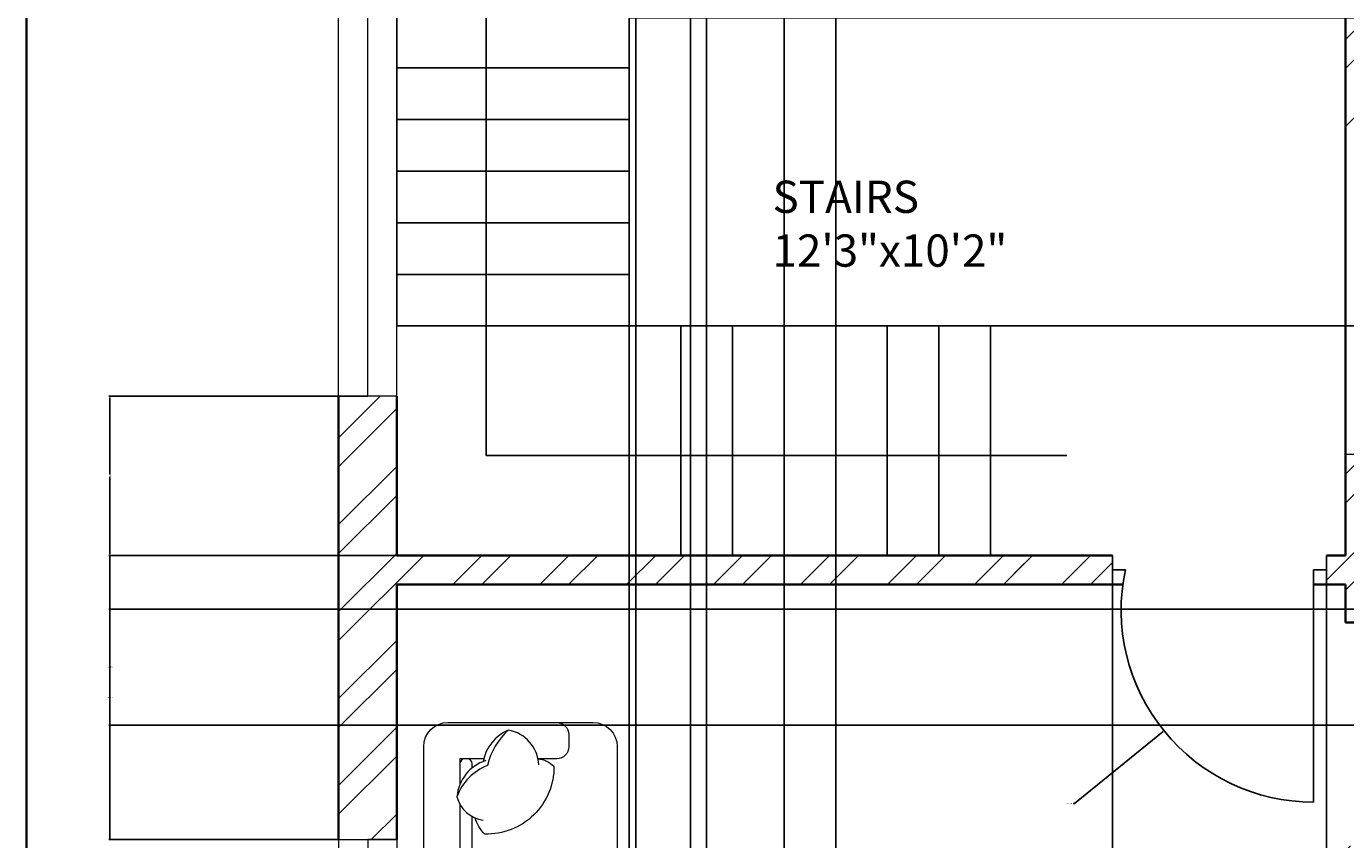
# Model space of a CAD drawing. Units: inches. Extents: x 2529 to 3014, y 1203 to 2262.
# Tile 3 of 13: x 2529 to 2733, y 1747 to 1873. Entities that reach past the tile are written whole.
import ezdxf

# ---------------------------------------------------------------- set-up
doc = ezdxf.new("R2010")
doc.units = ezdxf.units.IN
for name, color, linetype, lineweight in [('A-ANNO-DIMS', 2, 'Continuous', 18), ('A-ANNO-TTLB', 7, 'Continuous', 35), ('A-AREA-IDEN', 7, 'Continuous', 18), ('A-DOOR', 21, 'Continuous', 25), ('A-FLOR-STRS', 61, 'Continuous', 25), ('A-FURN', 8, 'Continuous', 18), ('A-GLAZ', 191, 'Continuous', 18), ('A-WALL', 7, 'Continuous', 35), ('A-WALL-PATT', 143, 'Continuous', 13)]:
    doc.layers.add(name, color=color, linetype=linetype, lineweight=lineweight)
doc.styles.get("Standard").update_dxf_attribs({"font": 'arial.ttf'})
doc.dimstyles.get("Standard").update_dxf_attribs({"dimtxt": 0.18, "dimasz": 0.18, "dimexe": 0.18, "dimexo": 0.0625, "dimgap": 0.09, "dimtad": 0, "dimtih": 1, "dimtoh": 1, "dimdec": 4, "dimzin": 0, "dimdsep": 46, "dimtxsty": 'Standard', "dimcen": 0.09, "dimadec": 0, "dimazin": 0, "dimtfac": 1, "dimtdec": 4, "dimtofl": 0, "dimtmove": 0, "dimatfit": 3, "dimfxl": 1, "dimtolj": 1, "dimtzin": 0, "dimarcsym": 0})

# ---------------------------------------------------------------- blocks, each defined once
blk = doc.blocks.new('WIN-60x9')
for p, q in [((0, 60), (9, 60)), ((0, 60), (0, 0)), ((9, 60), (4.5, 60)), ((4.5, 60), (4.5, 0)), ((9, 60), (9, 0)), ((4.5, 0), (0, 0)), ((0, 0), (9, 0))]:
    blk.add_line(p, q)
blk = doc.blocks.new('*D23')
at = {"layer": 'A-ANNO-DIMS', "color": 0, "lineweight": -2, "transparency": 16777216}
for p, q in [((2585.99, 1791), (2541.45, 1791)), ((2541.63, 1790.82), (2541.63, 1769.16)), ((2541.63, 1747.13), (2541.63, 1768.79)), ((2576.99, 1746.95), (2541.45, 1746.95))]:
    blk.add_line(p, q, dxfattribs=at)
at = {"layer": 'A-ANNO-DIMS', "color": 0, "transparency": 16777216}
for points in [[(2541.6, 1790.82), (2541.66, 1790.82), (2541.63, 1791)], [(2541.6, 1747.13), (2541.66, 1747.13), (2541.63, 1746.95)]]:
    blk.add_solid(points, dxfattribs=at)
at = {"layer": 'Defpoints', "color": 0, "transparency": 16777216}
for p in [(2541.63, 1791), (2586.06, 1791), (2577.06, 1746.95)]:
    blk.add_point(p, dxfattribs=at)
at = {"layer": 'A-ANNO-DIMS', "color": 0, "transparency": 16777216, "insert": (2541.63, 1768.98), "char_height": 0.18, "attachment_point": 5}
blk.add_mtext('\\A1;44.055', dxfattribs=at)
blk = doc.blocks.new('*D24')
at = {"layer": 'A-ANNO-DIMS', "color": 0, "lineweight": -2, "transparency": 16777216}
for p, q in [((2576.99, 1815.67), (2541.45, 1815.67)), ((2541.63, 1815.49), (2541.63, 1803.52)), ((2541.63, 1791.18), (2541.63, 1803.16)), ((2585.99, 1791), (2541.45, 1791))]:
    blk.add_line(p, q, dxfattribs=at)
at = {"layer": 'A-ANNO-DIMS', "color": 0, "transparency": 16777216}
for points in [[(2541.6, 1815.49), (2541.66, 1815.49), (2541.63, 1815.67)], [(2541.6, 1791.18), (2541.66, 1791.18), (2541.63, 1791)]]:
    blk.add_solid(points, dxfattribs=at)
at = {"layer": 'Defpoints', "color": 0, "transparency": 16777216}
for p in [(2541.63, 1815.67), (2577.06, 1815.67), (2586.06, 1791)]:
    blk.add_point(p, dxfattribs=at)
at = {"layer": 'A-ANNO-DIMS', "color": 0, "transparency": 16777216, "insert": (2541.63, 1803.34), "char_height": 0.18, "attachment_point": 5}
blk.add_mtext('\\A1;24.67', dxfattribs=at)
blk = doc.blocks.new('*D32')
at = {"layer": 'A-ANNO-DIMS', "color": 0, "lineweight": -2, "transparency": 16777216}
for p, q in [((2586.06, 1826.63), (2586.06, 2243.11)), ((2586.24, 2242.93), (2603.84, 2242.93)), ((2621.88, 2242.93), (2604.27, 2242.93)), ((2622.06, 1826.63), (2622.06, 2243.11))]:
    blk.add_line(p, q, dxfattribs=at)
at = {"layer": 'A-ANNO-DIMS', "color": 0, "transparency": 16777216}
for points in [[(2586.24, 2242.96), (2586.24, 2242.9), (2586.06, 2242.93)], [(2621.88, 2242.96), (2621.88, 2242.9), (2622.06, 2242.93)]]:
    blk.add_solid(points, dxfattribs=at)
at = {"layer": 'Defpoints', "color": 0, "transparency": 16777216}
for p in [(2622.06, 2242.93), (2586.06, 1826.57), (2622.06, 1826.57)]:
    blk.add_point(p, dxfattribs=at)
at = {"layer": 'A-ANNO-DIMS', "color": 0, "transparency": 16777216, "insert": (2604.06, 2242.93), "char_height": 0.18, "attachment_point": 5}
blk.add_mtext('\\A1;36', dxfattribs=at)
blk = doc.blocks.new('*D53')
at = {"layer": 'A-ANNO-DIMS', "color": 0, "lineweight": -2, "transparency": 16777216}
for p, q in [((2696.93, 1790.94), (2696.93, 1483.77)), ((2730.09, 1790.94), (2730.09, 1483.77)), ((2697.11, 1483.95), (2713.11, 1483.95)), ((2729.91, 1483.95), (2713.9, 1483.95))]:
    blk.add_line(p, q, dxfattribs=at)
at = {"layer": 'A-ANNO-DIMS', "color": 0, "transparency": 16777216}
for points in [[(2697.11, 1483.98), (2697.11, 1483.92), (2696.93, 1483.95)], [(2729.91, 1483.98), (2729.91, 1483.92), (2730.09, 1483.95)]]:
    blk.add_solid(points, dxfattribs=at)
at = {"layer": 'Defpoints', "color": 0, "transparency": 16777216}
for p in [(2696.93, 1791), (2730.09, 1791), (2730.09, 1483.95)]:
    blk.add_point(p, dxfattribs=at)
at = {"layer": 'A-ANNO-DIMS', "color": 0, "transparency": 16777216, "insert": (2713.51, 1483.95), "char_height": 0.18, "attachment_point": 5}
blk.add_mtext('\\A1;33.15', dxfattribs=at)
blk = doc.blocks.new('*D62')
at = {"layer": 'A-ANNO-DIMS', "color": 0, "lineweight": -2, "transparency": 16777216}
for p, q in [((2904.99, 1782.69), (2541.45, 1782.69)), ((2541.63, 1782.51), (2541.63, 1773.88)), ((2541.63, 1764.89), (2541.63, 1773.52)), ((2904.99, 1764.71), (2541.45, 1764.71))]:
    blk.add_line(p, q, dxfattribs=at)
at = {"layer": 'A-ANNO-DIMS', "color": 0, "transparency": 16777216}
for points in [[(2541.6, 1782.51), (2541.66, 1782.51), (2541.63, 1782.69)], [(2541.6, 1764.89), (2541.66, 1764.89), (2541.63, 1764.71)]]:
    blk.add_solid(points, dxfattribs=at)
at = {"layer": 'Defpoints', "color": 0, "transparency": 16777216}
for p in [(2905.06, 1782.69), (2541.63, 1764.71), (2905.06, 1764.71)]:
    blk.add_point(p, dxfattribs=at)
at = {"layer": 'A-ANNO-DIMS', "color": 0, "transparency": 16777216, "insert": (2541.63, 1773.7), "char_height": 0.18, "attachment_point": 5}
blk.add_mtext('\\A1;17.983', dxfattribs=at)
blk = doc.blocks.new('*D65')
at = {"layer": 'A-ANNO-DIMS', "color": 0, "lineweight": -2, "transparency": 16777216}
for p, q in [((2646.06, 1874.24), (2646.06, 1483.77)), ((2654.06, 1874.24), (2654.06, 1483.77)), ((2646.24, 1483.95), (2649.91, 1483.95)), ((2653.88, 1483.95), (2650.2, 1483.95))]:
    blk.add_line(p, q, dxfattribs=at)
at = {"layer": 'A-ANNO-DIMS', "color": 0, "transparency": 16777216}
for points in [[(2646.24, 1483.98), (2646.24, 1483.92), (2646.06, 1483.95)], [(2653.88, 1483.98), (2653.88, 1483.92), (2654.06, 1483.95)]]:
    blk.add_solid(points, dxfattribs=at)
at = {"layer": 'Defpoints', "color": 0, "transparency": 16777216}
for p in [(2646.06, 1874.3), (2654.06, 1874.3), (2654.06, 1483.95)]:
    blk.add_point(p, dxfattribs=at)
at = {"layer": 'A-ANNO-DIMS', "color": 0, "transparency": 16777216, "insert": (2650.06, 1483.95), "char_height": 0.18, "attachment_point": 5}
blk.add_mtext('\\A1;8', dxfattribs=at)
blk = doc.blocks.new('*D68')
at = {"layer": 'A-ANNO-DIMS', "color": 0, "lineweight": -2, "transparency": 16777216}
for p, q in [((2622.12, 1874.3), (3007.66, 1874.3)), ((3007.48, 1874.12), (3007.48, 1850.62)), ((3007.48, 1826.75), (3007.48, 1850.25)), ((2622.12, 1826.57), (3007.66, 1826.57))]:
    blk.add_line(p, q, dxfattribs=at)
at = {"layer": 'A-ANNO-DIMS', "color": 0, "transparency": 16777216}
for points in [[(3007.45, 1874.12), (3007.51, 1874.12), (3007.48, 1874.3)], [(3007.45, 1826.75), (3007.51, 1826.75), (3007.48, 1826.57)]]:
    blk.add_solid(points, dxfattribs=at)
at = {"layer": 'Defpoints', "color": 0, "transparency": 16777216}
for p in [(2622.06, 1874.3), (3007.48, 1874.3), (2622.06, 1826.57)]:
    blk.add_point(p, dxfattribs=at)
at = {"layer": 'A-ANNO-DIMS', "color": 0, "transparency": 16777216, "insert": (3007.48, 1850.43), "char_height": 0.18, "attachment_point": 5}
blk.add_mtext('\\A1;47.735', dxfattribs=at)
blk = doc.blocks.new('*D71')
at = {"layer": 'A-ANNO-DIMS', "color": 0, "lineweight": -2, "transparency": 16777216}
for p, q in [((2623.09, 2159.68), (2623.09, 1483.77)), ((2631.58, 2159.68), (2631.58, 1483.77)), ((2623.27, 1483.95), (2626.94, 1483.95)), ((2631.4, 1483.95), (2627.73, 1483.95))]:
    blk.add_line(p, q, dxfattribs=at)
at = {"layer": 'A-ANNO-DIMS', "color": 0, "transparency": 16777216}
for points in [[(2623.27, 1483.98), (2623.27, 1483.92), (2623.09, 1483.95)], [(2631.4, 1483.98), (2631.4, 1483.92), (2631.58, 1483.95)]]:
    blk.add_solid(points, dxfattribs=at)
at = {"layer": 'Defpoints', "color": 0, "transparency": 16777216}
for p in [(2623.09, 2159.75), (2631.58, 2159.75), (2631.58, 1483.95)]:
    blk.add_point(p, dxfattribs=at)
at = {"layer": 'A-ANNO-DIMS', "color": 0, "transparency": 16777216, "insert": (2627.33, 1483.95), "char_height": 0.18, "attachment_point": 5}
blk.add_mtext('\\A1;8.484', dxfattribs=at)
blk = doc.blocks.new('*D74')
at = {"layer": 'A-ANNO-DIMS', "color": 0, "lineweight": -2, "transparency": 16777216}
for p, q in [((2622.06, 2135.91), (2622.06, 1483.77)), ((2634.06, 2135.91), (2634.06, 1483.77)), ((2622.24, 1483.95), (2627.6, 1483.95)), ((2633.88, 1483.95), (2628.51, 1483.95))]:
    blk.add_line(p, q, dxfattribs=at)
at = {"layer": 'A-ANNO-DIMS', "color": 0, "transparency": 16777216}
for points in [[(2622.24, 1483.98), (2622.24, 1483.92), (2622.06, 1483.95)], [(2633.88, 1483.98), (2633.88, 1483.92), (2634.06, 1483.95)]]:
    blk.add_solid(points, dxfattribs=at)
at = {"layer": 'Defpoints', "color": 0, "transparency": 16777216}
for p in [(2622.06, 2135.98), (2634.06, 2135.98), (2634.06, 1483.95)]:
    blk.add_point(p, dxfattribs=at)
at = {"layer": 'A-ANNO-DIMS', "color": 0, "transparency": 16777216, "insert": (2628.06, 1483.95), "char_height": 0.18, "attachment_point": 5}
blk.add_mtext('\\A1;12.002', dxfattribs=at)
blk = doc.blocks.new('*D83')
at = {"layer": 'A-ANNO-DIMS', "color": 0, "lineweight": -2, "transparency": 16777216}
for p, q in [((2728, 1782.56), (2728.18, 1782.56)), ((2728.09, 1782.47), (2728.09, 1782.65)), ((2691.03, 1752.55), (2704.78, 1763.69)), ((2690.85, 1752.55), (2691.03, 1752.55))]:
    blk.add_line(p, q, dxfattribs=at)
at = {"layer": 'A-ANNO-DIMS', "color": 0, "transparency": 16777216}
blk.add_solid([(2704.76, 1763.71), (2704.8, 1763.66), (2704.92, 1763.8)], dxfattribs=at)
at = {"layer": 'Defpoints', "color": 0, "transparency": 16777216}
for p in [(2728.09, 1782.56), (2704.92, 1763.8)]:
    blk.add_point(p, dxfattribs=at)
at = {"layer": 'A-ANNO-DIMS', "color": 0, "transparency": 16777216, "insert": (2690.3, 1752.55), "char_height": 0.18, "attachment_point": 5}
blk.add_mtext('\\A1;R29.804', dxfattribs=at)

msp = doc.modelspace()

# ---------------------------------------------------------------- hatches: boundary and pattern name
at = {"layer": 'A-WALL-PATT'}
h = msp.add_hatch(dxfattribs=at)
h.set_pattern_fill('ANSI32', color=256)
h.paths.add_polyline_path([(2686.5554, 2106.5032), (2622.0554, 2106.5032), (2622.0554, 2109.2964), (2617.4223, 2109.2964), (2613.0554, 2109.2964), (2613.0554, 2106.5032), (2577.0554, 2106.5032), (2577.0554, 2092.6918), (2586.0554, 2092.6918), (2586.0554, 2102.0032), (2682.0554, 2102.0032), (2682.0554, 2099.9833), (2686.5554, 2099.9833), (2686.5554, 2102.0032)])
h.paths.add_polyline_path([(2695.2249, 2054.0032), (2686.5554, 2054.0032), (2686.5554, 2080.2316), (2684.3054, 2080.2316), (2682.0554, 2080.2316), (2682.0554, 2054.0032), (2586.0554, 2054.0032), (2586.0554, 2068.6918), (2577.0554, 2068.6918), (2577.0554, 2019.1229), (2586.0554, 2019.1229), (2586.0554, 2049.5032), (2695.2249, 2049.5032)])
h.paths.add_polyline_path([(2737.5554, 2049.5032), (2866.5554, 2049.5032), (2866.5554, 2045.0233), (2871.0554, 2045.0233), (2871.0554, 2049.5032), (2871.0554, 2172.5032), (2866.5554, 2172.5032), (2829.1265, 2172.5032), (2829.1265, 2168.0032), (2866.5554, 2168.0032), (2866.5554, 2054.0032), (2737.5554, 2054.0032), (2737.5554, 2056.4892), (2735.3054, 2056.4892), (2733.0554, 2056.4892), (2733.0554, 2049.5032), (2733.0554, 1917.5032), (2733.0554, 1913.0032), (2871.0554, 1913.0032), (2871.0554, 1924.9149), (2868.8054, 1924.9149), (2866.5554, 1924.9149), (2866.5554, 1917.5032), (2737.5554, 1917.5032)], flags=17)
h.paths.add_polyline_path([(2972.0554, 2207.5032), (2613.0554, 2207.5032), (2613.0554, 2205.5032), (2613.0554, 2188.9366), (2622.0554, 2188.9366), (2622.0554, 2198.5032), (2733.0554, 2198.5032), (2733.0554, 2084.8053), (2735.3054, 2084.8053), (2737.5554, 2084.8053), (2737.5554, 2168.0032), (2769.1265, 2168.0032), (2769.1265, 2170.2532), (2769.1265, 2172.5032), (2737.5554, 2172.5032), (2737.5554, 2198.5032), (2963.0554, 2198.5032), (2963.0554, 2093.5032), (2912.0586, 2093.5032), (2912.0586, 2089.0032), (2918.5554, 2089.0032), (2918.5554, 2031.8749), (2923.0554, 2031.8749), (2923.0554, 2089.0032), (2963.0554, 2089.0032), (2963.0554, 2010.0032), (2923.0554, 2010.0032), (2923.0554, 2011.9417), (2918.5554, 2011.9417), (2918.5554, 2003.1338), (2923.0554, 2003.1338), (2923.0554, 2005.5032), (2963.0554, 2005.5032), (2963.0554, 1917.5032), (2963.0554, 1691.0776), (2972.0554, 1691.0776), (2972.0554, 1917.5032)])
h.paths.add_polyline_path([(2963.0554, 1945.5032), (2923.0554, 1945.5032), (2923.0554, 1983.0571), (2920.8054, 1983.0571), (2918.5554, 1983.0571), (2918.5554, 1941.0032), (2963.0554, 1941.0032)], flags=17)
h.paths.add_polyline_path([(2930.3679, 1788.7532), (2930.3679, 1791.0032), (2894.8637, 1791.0032), (2894.8637, 1786.5032), (2900.5554, 1786.5032), (2900.5554, 1784.6931), (2905.0554, 1784.6931), (2905.0554, 1786.5032), (2930.3679, 1786.5032)], flags=17)
h.paths.add_polyline_path([(2963.0554, 1791.0032), (2954.3679, 1791.0032), (2954.3679, 1786.5032), (2963.0554, 1786.5032)], flags=17)
h.paths.add_polyline_path([(2871.0554, 1853.0032), (2919.0554, 1853.0032), (2919.0554, 1847.0972), (2923.5554, 1847.0972), (2923.5554, 1853.0032), (2923.5554, 1857.5032), (2871.0554, 1857.5032), (2871.0554, 1871.7024), (2866.5554, 1871.7024), (2866.5554, 1791.0032), (2737.5554, 1791.0032), (2737.5554, 1806.6712), (2735.3054, 1806.6712), (2733.0554, 1806.6712), (2733.0554, 1791.0032), (2733.0554, 1786.5032), (2733.0554, 1780.6235), (2737.5554, 1780.6235), (2737.5554, 1786.5032), (2872.8745, 1786.5032), (2872.8745, 1788.7532), (2872.8745, 1791.0032), (2871.0554, 1791.0032)], flags=17)
h.paths.add_polyline_path([(2844.0554, 1734.0032), (2848.2652, 1734.0032), (2848.2652, 1738.5032), (2800.0167, 1738.5032), (2800.0167, 1734.0032), (2839.5554, 1734.0032), (2839.5554, 1582.5032), (2792.3334, 1582.5032), (2792.3334, 1573.5032), (2871.4433, 1573.5032), (2871.4433, 1578.0032), (2871.4433, 1582.5032), (2844.0554, 1582.5032)])
h.paths.add_polyline_path([(2972.0554, 1631.0776), (2963.0554, 1631.0776), (2963.0554, 1582.5032), (2931.4433, 1582.5032), (2931.4433, 1573.5032), (2972.0554, 1573.5032)])
h.paths.add_polyline_path([(2756.3334, 1582.5032), (2737.5554, 1582.5032), (2737.5554, 1734.0032), (2744.3201, 1734.0032), (2744.3201, 1738.5032), (2737.5554, 1738.5032), (2737.5554, 1746.0094), (2733.0554, 1746.0094), (2733.0554, 1738.5032), (2733.0554, 1612.5032), (2728.2475, 1612.5032), (2728.2475, 1603.5032), (2733.0554, 1603.5032), (2733.0554, 1582.5032), (2733.0554, 1573.5032), (2756.3334, 1573.5032), (2756.3334, 1578.0032)])
h.paths.add_polyline_path([(2695.7662, 1612.5032), (2658.4771, 1612.5032), (2658.4771, 1603.5032), (2695.7662, 1603.5032), (2695.7662, 1608.0032)])
h.paths.add_polyline_path([(2586.0554, 1686.9483), (2577.0554, 1686.9483), (2577.0554, 1603.5032), (2598.4771, 1603.5032), (2598.4771, 1608.0032), (2598.4771, 1612.5032), (2586.0554, 1612.5032)])
h.paths.add_polyline_path([(2683.2727, 1791.0032), (2586.0554, 1791.0032), (2586.0554, 1815.6736), (2581.5554, 1815.6736), (2577.0554, 1815.6736), (2577.0554, 1746.9483), (2586.0554, 1746.9483), (2586.0554, 1786.5032), (2683.2727, 1786.5032)])
h.paths.add_polyline_path([(2586.0554, 1959.1229), (2577.0554, 1959.1229), (2577.0554, 1875.6736), (2586.0554, 1875.6736), (2586.0554, 1913.0032), (2683.2727, 1913.0032), (2683.2727, 1917.5032), (2586.0554, 1917.5032)])
h = msp.add_hatch(dxfattribs=at)
h.set_pattern_fill('ANSI32', color=256)
h.paths.add_polyline_path([(2737.5554, 1786.5032), (2872.8745, 1786.5032), (2872.8745, 1788.7532), (2872.8745, 1791.0032), (2871.0554, 1791.0032), (2871.0554, 1853.0032), (2919.0554, 1853.0032), (2919.0554, 1847.0972), (2923.5554, 1847.0972), (2923.5554, 1853.0032), (2923.5554, 1857.5032), (2871.0554, 1857.5032), (2871.0554, 1871.7024), (2866.5554, 1871.7024), (2866.5554, 1791.0032), (2737.5554, 1791.0032), (2737.5554, 1806.6712), (2735.3054, 1806.6712), (2733.0554, 1806.6712), (2733.0554, 1791.0032), (2730.085, 1791.0032), (2730.085, 1786.5032), (2733.0554, 1786.5032), (2733.0554, 1780.6235), (2737.5554, 1780.6235)])
h.paths.add_polyline_path([(2737.5554, 1880.8133), (2735.3054, 1880.8133), (2733.0554, 1880.8133), (2733.0554, 1854.6712), (2737.5554, 1854.6712)])
h.paths.add_polyline_path([(2695.1228, 1915.2532), (2695.1228, 1917.5032), (2586.0554, 1917.5032), (2586.0554, 1959.1229), (2577.0554, 1959.1229), (2577.0554, 1875.6736), (2586.0554, 1875.6736), (2586.0554, 1913.0032), (2695.1228, 1913.0032)])
h = msp.add_hatch(dxfattribs=at)
h.set_pattern_fill('ANSI32', color=256)
h.paths.add_polyline_path([(2696.9325, 1791.0032), (2586.0554, 1791.0032), (2586.0554, 1815.6736), (2581.5554, 1815.6736), (2577.0554, 1815.6736), (2577.0554, 1746.9483), (2586.0554, 1746.9483), (2586.0554, 1786.5032), (2696.9325, 1786.5032)])
h.paths.add_polyline_path([(2872.8745, 1791.0032), (2871.0554, 1791.0032), (2871.0554, 1853.0032), (2919.0554, 1853.0032), (2919.0554, 1847.0972), (2923.5554, 1847.0972), (2923.5554, 1853.0032), (2923.5554, 1857.5032), (2871.0554, 1857.5032), (2871.0554, 1871.7024), (2866.5554, 1871.7024), (2866.5554, 1791.0032), (2737.5554, 1791.0032), (2737.5554, 1806.6712), (2735.3054, 1806.6712), (2733.0554, 1806.6712), (2733.0554, 1791.0032), (2730.085, 1791.0032), (2730.085, 1786.5032), (2733.0554, 1786.5032), (2733.0554, 1780.6235), (2737.5554, 1780.6235), (2737.5554, 1786.5032), (2872.8745, 1786.5032), (2872.8745, 1788.7532)])

# ---------------------------------------------------------------- linework, layer by layer
at = {"layer": 'A-ANNO-TTLB'}
msp.add_lwpolyline([(2528.6765, 2261.8165), (3013.6003, 2261.8165), (3013.6003, 1455.1523), (2528.6765, 1455.1523)], close=True, dxfattribs=at)
at = {"layer": 'A-DOOR'}
for p, q in [((2696.9325, 1786.5032), (2696.9325, 1791.0032)), ((2696.9325, 1791.0032), (2696.9325, 1788.7532)), ((2730.085, 1791.0032), (2730.085, 1786.5032)), ((2696.9325, 1788.7532), (2698.9325, 1788.7532)), ((2730.085, 1788.7532), (2728.085, 1788.7532)), ((2728.085, 1788.7532), (2728.085, 1752.7532)), ((2730.085, 1786.5032), (2730.085, 1788.7532))]:
    msp.add_line(p, q, dxfattribs=at)
msp.add_arc((2728.085, 1782.557), 29.8038, 168.000705, 270, dxfattribs=at)
at = {"layer": 'A-FLOR-STRS'}
for p, q in [((2599.8977, 1806.4779), (2599.8977, 1901.5876)), ((2622.0554, 1826.5675), (2622.0554, 1874.3024)), ((2622.0554, 1866.5675), (2586.0554, 1866.5675)), ((2622.0554, 1858.5675), (2586.0554, 1858.5675)), ((2622.0554, 1850.5675), (2586.0554, 1850.5675)), ((2622.0554, 1842.5675), (2586.0554, 1842.5675)), ((2622.0554, 1834.5675), (2586.0554, 1834.5675)), ((2622.0554, 1826.5675), (2586.0554, 1826.5675)), ((2622.0554, 1791.0032), (2622.0554, 1826.5675)), ((2678.0554, 1826.5675), (2622.0554, 1826.5675)), ((2630.0554, 1791.0032), (2630.0554, 1826.5675)), ((2638.0554, 1791.0032), (2638.0554, 1826.5675)), ((2646.0554, 1791.0032), (2646.0554, 1826.5675)), ((2654.0554, 1791.0032), (2654.0554, 1826.5675)), ((2662.0554, 1791.0032), (2662.0554, 1826.5675)), ((2670.0554, 1791.0032), (2670.0554, 1826.5675)), ((2678.0554, 1791.0032), (2678.0554, 1826.5675)), ((2689.8493, 1806.4779), (2599.8977, 1806.4779))]:
    msp.add_line(p, q, dxfattribs=at)
at = {"layer": 'A-FURN', "ltscale": 0.03}
msp.add_lwpolyline([(2620.206, 1738.8743, -0.41421356), (2618.3324, 1737.0007, -0.41421356), (2620.206, 1735.1271), (2620.206, 1712.6442, -0.41421356), (2616.4588, 1708.897), (2593.9759, 1708.897, -0.41421356), (2590.2287, 1712.6442), (2590.2287, 1761.3573, -0.41421356), (2593.9759, 1765.1045), (2616.4588, 1765.1045, -0.41421356), (2620.206, 1761.3573), (2620.206, 1738.8743, -0.41421356), (2618.3324, 1737.0007, -0.41421356), (2620.206, 1735.1271)], format="xyb", dxfattribs=at)
at = {"layer": 'A-FURN'}
for points in [[(2603.326, 1763.912, 0.14772988), (2600.1061, 1758.4361, 0.21334276), (2595.3835, 1753.6044, 0.17866181)], [(2608.0486, 1758.5435, 0.35677236), (2603.326, 1763.912, 0.24954205), (2599.4342, 1759.0476, -9.61688035)], [(2610.8381, 1765.1045, -0.41421356), (2612.7117, 1763.2309), (2612.7117, 1761.3573, -0.41421356), (2610.8381, 1759.4837), (2607.9352, 1759.4837)], [(2599.8495, 1759.1926, 0.30666349), (2595.3835, 1753.6044, 0.30632997), (2599.4621, 1749.9538, -0.87284716)], [(2597.723, 1758.0539), (2597.723, 1758.7343, 0.41421356), (2596.9736, 1759.4837), (2596.5989, 1759.4837, 0.41421356), (2595.8494, 1758.7343)], [(2595.8494, 1758.7343), (2595.8494, 1755.5422, 0.41421356)], [(2607.9344, 1759.4878, -0.16554063), (2610.4099, 1758.3287, -0.42598917), (2599.6768, 1747.8063, -0.12152332), (2598.1974, 1750.3041, 7.11546429)], [(2595.8494, 1752.4253), (2595.8494, 1737.7502, 0.41421356), (2596.5989, 1737.0007), (2596.9736, 1737.0007, 0.41421356), (2597.723, 1737.7502), (2597.723, 1750.5387, 0.41421356)]]:
    msp.add_lwpolyline(points, format="xyb", dxfattribs=at)
for points in [[(2599.5315, 1759.4837), (2595.8494, 1759.4837), (2595.8494, 1755.5422)], [(2595.8494, 1752.4253), (2595.8494, 1731.6691)]]:
    msp.add_lwpolyline(points, dxfattribs=at)
at = {"layer": 'A-GLAZ'}
for p, q in [((2733.0554, 1854.6712), (2733.0554, 1806.6712)), ((2733.0554, 1806.6712), (2737.5554, 1806.6712))]:
    msp.add_line(p, q, dxfattribs=at)
at = {"layer": 'A-WALL'}
for p, q in [((2733.0554, 1880.8133), (2733.0554, 1806.6712)), ((2577.0554, 1815.6736), (2577.0554, 1746.9483)), ((2586.0554, 1815.6736), (2586.0554, 1791.0032)), ((2733.0554, 1806.6712), (2733.0554, 1791.0032)), ((2586.0554, 1791.0032), (2696.9325, 1791.0032)), ((2730.085, 1791.0032), (2733.0554, 1791.0032)), ((2586.0554, 1786.5032), (2698.5437, 1786.5032)), ((2586.0554, 1786.5032), (2586.0554, 1746.9483)), ((2586.0554, 1786.5032), (2586.0554, 1746.9483)), ((2728.085, 1786.5032), (2733.0554, 1786.5032)), ((2733.0554, 1786.5032), (2733.0554, 1780.6235)), ((2733.0554, 1780.6235), (2737.5554, 1780.6235))]:
    msp.add_line(p, q, dxfattribs=at)

# ---------------------------------------------------------------- block references
at = {"layer": 'A-GLAZ', "rotation": 180}
msp.add_blockref('WIN-60x9', (2586.0557, 1875.6735), dxfattribs=at)
at = {"layer": 'A-GLAZ'}
msp.add_blockref('WIN-60x9', (2577.055, 1686.9484), dxfattribs=at)

# ---------------------------------------------------------------- texts
at = {"layer": 'A-AREA-IDEN', "insert": (2644.2721, 1849.088), "char_height": 5, "attachment_point": 1}
msp.add_mtext_dynamic_manual_height_columns('STAIRS\\P12\'3"x10\'2"', width=55.718606, gutter_width=12.5, heights=[0], dxfattribs=at)

# ---------------------------------------------------------------- dimensions: what is measured, and where the dimension line sits
at = {"layer": 'A-ANNO-DIMS'}
for base, p1, p2, override, picture, middle in [((2622.0554, 2242.9282), (2586.0554, 1826.5675), (2622.0554, 1826.5675), {"dimdec": 0, "dimlfac": 1, "dimrnd": 0, "dimzin": 0, "dimdsep": 46, "dimlunit": 2}, '*D32', (2604.0554, 2242.9282)), ((2631.5753, 1483.9492), (2623.0916, 2159.7466), (2631.5753, 2159.7466), {"dimdec": 3, "dimlfac": 1, "dimrnd": 0, "dimzin": 0, "dimdsep": 46, "dimlunit": 2}, '*D71', (2627.3335, 1483.9492)), ((2634.0572, 1483.9492), (2622.0554, 2135.9767), (2634.0572, 2135.9767), {"dimdec": 3, "dimlfac": 1, "dimrnd": 0, "dimzin": 0, "dimdsep": 46, "dimlunit": 2}, '*D74', (2628.0563, 1483.9492)), ((2654.0554, 1483.9492), (2646.0554, 1874.3024), (2654.0554, 1874.3024), {"dimdec": 0, "dimlfac": 1, "dimrnd": 0, "dimzin": 0, "dimdsep": 46, "dimlunit": 2}, '*D65', (2650.0554, 1483.9492)), ((2730.085, 1483.9492), (2696.9325, 1791.0032), (2730.085, 1791.0032), {"dimdec": 2, "dimlfac": 1, "dimrnd": 0, "dimzin": 0, "dimdsep": 46, "dimlunit": 2}, '*D53', (2713.5087, 1483.9492))]:
    dim = msp.add_linear_dim(base=base, p1=p1, p2=p2, dimstyle='Standard', override=override, dxfattribs=at)
    dim.commit()
    dim.dimension.update_dxf_attribs({"geometry": picture, "text_midpoint": middle})
for base, p1, p2, override, picture, middle in [((3007.4804, 1874.3024), (2622.0554, 1826.5675), (2622.0554, 1874.3024), {"dimdec": 3, "dimlfac": 1, "dimrnd": 0, "dimzin": 0, "dimdsep": 46, "dimlunit": 2}, '*D68', (3007.4804, 1850.435)), ((2541.6304, 1815.6736), (2586.0554, 1791.0032), (2577.0554, 1815.6736), {"dimdec": 2, "dimlfac": 1, "dimrnd": 0, "dimzin": 0, "dimdsep": 46, "dimlunit": 2}, '*D24', (2541.6304, 1803.3384)), ((2541.6304, 1791.0032), (2577.0554, 1746.9483), (2586.0554, 1791.0032), {"dimdec": 3, "dimlfac": 1, "dimrnd": 0, "dimzin": 0, "dimdsep": 46, "dimlunit": 2}, '*D23', (2541.6304, 1768.9757)), ((2541.6304, 1764.7097), (2905.0554, 1782.6931), (2905.0554, 1764.7097), {"dimdec": 3, "dimlfac": 1, "dimrnd": 0, "dimzin": 0, "dimdsep": 46, "dimlunit": 2}, '*D62', (2541.6304, 1773.7014))]:
    dim = msp.add_linear_dim(base=base, p1=p1, p2=p2, angle=90, dimstyle='Standard', override=override, dxfattribs=at)
    dim.commit()
    dim.dimension.update_dxf_attribs({"geometry": picture, "text_midpoint": middle})
dim = msp.add_radius_dim(center=(2728.085, 1782.557), mpoint=(2704.923, 1763.801), dimstyle='Standard', override={"dimdec": 3, "dimlfac": 1, "dimrnd": 0, "dimzin": 0, "dimdsep": 46, "dimlunit": 2}, dxfattribs=at)
dim.commit()
dim.dimension.update_dxf_attribs({"geometry": '*D83', "text_midpoint": (2690.2964, 1752.5474), "dimtype": 164})

doc.saveas('drawing.dxf')
